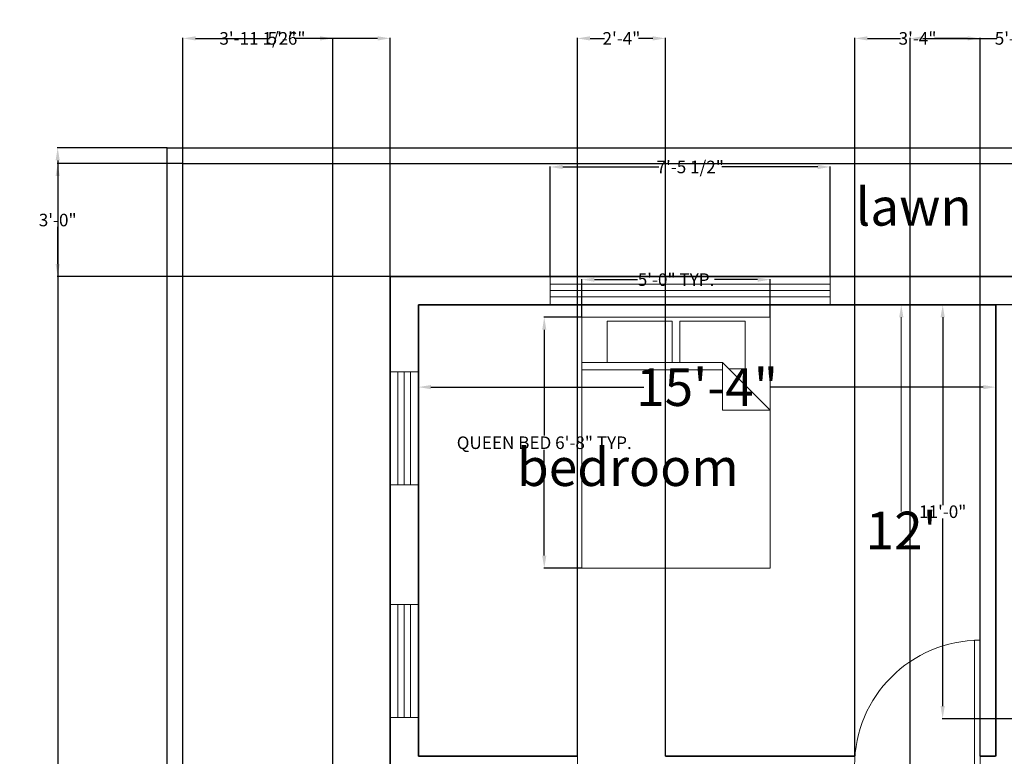
# Model space of a CAD drawing. Units: inches. Extents: x -346 to 220, y 97 to 877.
# Tile 3 of 4: x -346 to -32, y 642 to 877. Entities that reach past the tile are written whole.
import ezdxf

# ---------------------------------------------------------------- set-up
doc = ezdxf.new("R2010")
doc.units = ezdxf.units.IN
doc.header["$MEASUREMENT"] = 0
doc.layers.get('0').update_dxf_attribs({"color": 3})
for name, color, linetype, lineweight in [('A-AREA-IDEN', 130, 'Continuous', 25), ('A-FURN', 8, 'Continuous', 18), ('A-WALL', 7, 'Continuous', 35), ('C-PROP', 94, 'Continuous', 25), ('dim', 170, 'Continuous', 13), ('door', 20, 'Continuous', 18), ('window', 230, 'Continuous', 18)]:
    doc.layers.add(name, color=color, linetype=linetype, lineweight=lineweight)
doc.styles.get("Standard").update_dxf_attribs({"font": 'arial.ttf'})
doc.dimstyles.get("Standard").update_dxf_attribs({"dimtxt": 4, "dimasz": 4, "dimexe": 0.18, "dimexo": 0.0625, "dimgap": 0.09, "dimtad": 0, "dimtih": 1, "dimtoh": 1, "dimdec": 0, "dimzin": 0, "dimdsep": 46, "dimlunit": 3, "dimtxsty": 'Standard', "dimcen": 0.09, "dimadec": 0, "dimazin": 0, "dimtfac": 1, "dimtdec": 0, "dimtofl": 0, "dimtmove": 0, "dimatfit": 3, "dimfxl": 1, "dimtolj": 1, "dimtzin": 0, "dimarcsym": 0})

# ---------------------------------------------------------------- blocks, each defined once
blk = doc.blocks.new('*D1')
at = {"layer": 'Defpoints', "color": 0, "transparency": 16777216}
for p in [(-218.93, 785.75), (-34.93, 785.75), (-34.93, 759.47)]:
    blk.add_point(p, dxfattribs=at)
at = {"layer": 'dim', "color": 0, "lineweight": -2, "transparency": 16777216}
for p, q in [((-218.93, 785.68), (-218.93, 759.29)), ((-34.93, 785.68), (-34.93, 759.29)), ((-214.93, 759.47), (-147.06, 759.47)), ((-38.93, 759.47), (-106.79, 759.47))]:
    blk.add_line(p, q, dxfattribs=at)
at = {"layer": 'dim', "color": 0, "transparency": 16777216}
for points in [[(-214.93, 760.14), (-214.93, 758.8), (-218.93, 759.47)], [(-38.93, 760.14), (-38.93, 758.8), (-34.93, 759.47)]]:
    blk.add_solid(points, dxfattribs=at)
at = {"layer": 'dim', "color": 0, "transparency": 16777216, "insert": (-126.93, 759.47), "char_height": 4, "attachment_point": 5}
blk.add_mtext('\\A1;{\\H3x;15\'-4"}', dxfattribs=at)
blk = doc.blocks.new('*U18')
for p, q in [((0, 0), (0, -6)), ((-40, 0), (-40, -6))]:
    blk.add_line(p, q)
blk.add_lwpolyline([(0, 0), (0, 40), (-1.75, 40), (-1.75, 0)], close=True)
blk.add_arc((0, 0), 40, 90, 180)
blk = doc.blocks.new('Bed - Queen')
for p, q in [((0, -80.00003), (0, 0)), ((0, 0), (59.99999, 0)), ((59.99999, 0), (59.99999, -80.00003)), ((7.99999, -1.2), (28.79998, -1.2)), ((7.99999, -14.4), (7.99999, -1.2)), ((28.79998, -1.2), (28.79998, -14.4)), ((31.19999, -1.2), (51.99999, -1.2)), ((31.19999, -14.4), (31.19999, -1.2)), ((51.99999, -1.2), (51.99999, -16.4)), ((0, -14.4), (44.8, -14.4)), ((59.99999, -29.6), (44.8, -14.4)), ((44.8, -14.4), (44.8, -29.6)), ((44.8, -16.8), (0, -16.8)), ((51.99999, -16.4), (46.79936, -16.4)), ((44.8, -29.6), (59.99999, -29.6)), ((59.99999, -80.00003), (0, -80.00003))]:
    blk.add_line(p, q)
blk = doc.blocks.new('WIN-36x9-PLAN')
for p, q in [((2.5, 36), (2.5, 0)), ((4.5, 36), (4.5, 0)), ((6.5, 36), (6.5, 0))]:
    blk.add_line(p, q)
blk.add_lwpolyline([(0, 36), (9, 36), (9, 0), (0, 0)], close=True)
blk = doc.blocks.new('*D34')
at = {"layer": 'Defpoints', "color": 0, "transparency": 16777216}
for p in [(-178.82, 781.74), (-166.82, 781.74), (-166.82, 701.74)]:
    blk.add_point(p, dxfattribs=at)
at = {"layer": 'dim', "color": 0, "lineweight": -2, "transparency": 16777216}
for p, q in [((-166.88, 781.74), (-179, 781.74)), ((-178.82, 777.74), (-178.82, 744.02)), ((-178.82, 705.74), (-178.82, 739.46)), ((-166.88, 701.74), (-179, 701.74))]:
    blk.add_line(p, q, dxfattribs=at)
at = {"layer": 'dim', "color": 0, "transparency": 16777216}
for points in [[(-179.48, 777.74), (-178.15, 777.74), (-178.82, 781.74)], [(-179.48, 705.74), (-178.15, 705.74), (-178.82, 701.74)]]:
    blk.add_solid(points, dxfattribs=at)
at = {"layer": 'dim', "color": 0, "transparency": 16777216, "insert": (-178.82, 741.74), "char_height": 4, "attachment_point": 5}
blk.add_mtext('\\A1;QUEEN BED 6\'-8" TYP.', dxfattribs=at)
blk = doc.blocks.new('*D35')
at = {"layer": 'Defpoints', "color": 0, "transparency": 16777216}
for p in [(-106.82, 793.74), (-166.82, 781.74), (-106.82, 781.74)]:
    blk.add_point(p, dxfattribs=at)
at = {"layer": 'dim', "color": 0, "lineweight": -2, "transparency": 16777216}
for p, q in [((-166.82, 781.8), (-166.82, 793.92)), ((-106.82, 781.8), (-106.82, 793.92)), ((-162.82, 793.74), (-149.1, 793.74)), ((-110.82, 793.74), (-124.54, 793.74))]:
    blk.add_line(p, q, dxfattribs=at)
at = {"layer": 'dim', "color": 0, "transparency": 16777216}
for points in [[(-162.82, 794.4), (-162.82, 793.07), (-166.82, 793.74)], [(-110.82, 794.4), (-110.82, 793.07), (-106.82, 793.74)]]:
    blk.add_solid(points, dxfattribs=at)
at = {"layer": 'dim', "color": 0, "transparency": 16777216, "insert": (-136.82, 793.74), "char_height": 4, "attachment_point": 5}
blk.add_mtext('\\A1;5\'-0" TYP.', dxfattribs=at)
blk = doc.blocks.new('*D40')
at = {"layer": 'Defpoints', "color": 0, "transparency": 16777216}
for p in [(-93.45, 636.11), (-118, 632.43), (-93.45, 632.43)]:
    blk.add_point(p, dxfattribs=at)
at = {"layer": 'dim', "color": 0, "lineweight": -2, "transparency": 16777216}
for p, q in [((-118, 632.49), (-118, 636.29)), ((-114, 636.11), (-97.45, 636.11)), ((-93.45, 632.49), (-93.45, 636.29)), ((-93.45, 636.11), (-89.45, 636.11))]:
    blk.add_line(p, q, dxfattribs=at)
at = {"layer": 'dim', "color": 0, "transparency": 16777216}
for points in [[(-114, 636.78), (-114, 635.45), (-118, 636.11)], [(-97.45, 636.78), (-97.45, 635.45), (-93.45, 636.11)]]:
    blk.add_solid(points, dxfattribs=at)
at = {"layer": 'dim', "color": 0, "transparency": 16777216, "insert": (-63.43, 636.11), "char_height": 4, "attachment_point": 5}
blk.add_mtext('\\A1;BASIN 2\'-0 1/2" TYP.', dxfattribs=at)
blk = doc.blocks.new('*D49')
at = {"layer": 'Defpoints', "color": 0, "transparency": 16777216}
for p in [(-333.87, 835.75), (-298.95, 835.75), (-298.95, 138.35)]:
    blk.add_point(p, dxfattribs=at)
at = {"layer": 'dim', "color": 0, "lineweight": -2, "transparency": 16777216}
for p, q in [((-299.01, 835.75), (-334.05, 835.75)), ((-333.87, 831.75), (-333.87, 489.21)), ((-333.87, 142.35), (-333.87, 484.89)), ((-299.01, 138.35), (-334.05, 138.35))]:
    blk.add_line(p, q, dxfattribs=at)
at = {"layer": 'dim', "color": 0, "transparency": 16777216}
for points in [[(-334.54, 831.75), (-333.21, 831.75), (-333.87, 835.75)], [(-334.54, 142.35), (-333.21, 142.35), (-333.87, 138.35)]]:
    blk.add_solid(points, dxfattribs=at)
at = {"layer": 'dim', "color": 0, "transparency": 16777216, "insert": (-333.87, 487.05), "char_height": 4, "attachment_point": 5}
blk.add_mtext('\\A1;58\'-1 1/2"', dxfattribs=at)
blk = doc.blocks.new('*D52')
at = {"layer": 'Defpoints', "color": 0, "transparency": 16777216}
for p in [(-246.23, 870.67), (-246.23, 242.75), (-293.95, 143.35)]:
    blk.add_point(p, dxfattribs=at)
at = {"layer": 'dim', "color": 0, "lineweight": -2, "transparency": 16777216}
for p, q in [((-293.95, 143.41), (-293.95, 870.85)), ((-289.95, 870.67), (-281.71, 870.67)), ((-250.23, 870.67), (-258.47, 870.67)), ((-246.23, 242.81), (-246.23, 870.85))]:
    blk.add_line(p, q, dxfattribs=at)
at = {"layer": 'dim', "color": 0, "transparency": 16777216}
for points in [[(-289.95, 871.34), (-289.95, 870), (-293.95, 870.67)], [(-250.23, 871.34), (-250.23, 870), (-246.23, 870.67)]]:
    blk.add_solid(points, dxfattribs=at)
at = {"layer": 'dim', "color": 0, "transparency": 16777216, "insert": (-270.09, 870.67), "char_height": 4, "attachment_point": 5}
blk.add_mtext('\\A1;3\'-11 1/2"', dxfattribs=at)
blk = doc.blocks.new('*D54')
at = {"layer": 'Defpoints', "color": 0, "transparency": 16777216}
for p in [(-293.95, 830.75), (-333.87, 794.75), (-227.93, 794.75)]:
    blk.add_point(p, dxfattribs=at)
at = {"layer": 'dim', "color": 0, "lineweight": -2, "transparency": 16777216}
for p, q in [((-294.01, 830.75), (-334.05, 830.75)), ((-333.87, 826.75), (-333.87, 814.88)), ((-333.87, 798.75), (-333.87, 810.61)), ((-227.99, 794.75), (-334.05, 794.75))]:
    blk.add_line(p, q, dxfattribs=at)
at = {"layer": 'dim', "color": 0, "transparency": 16777216}
for points in [[(-334.54, 826.75), (-333.21, 826.75), (-333.87, 830.75)], [(-334.54, 798.75), (-333.21, 798.75), (-333.87, 794.75)]]:
    blk.add_solid(points, dxfattribs=at)
at = {"layer": 'dim', "color": 0, "transparency": 16777216, "insert": (-333.87, 812.75), "char_height": 4, "attachment_point": 5}
blk.add_mtext('\\A1;3\'-0"', dxfattribs=at)
blk = doc.blocks.new('*D55')
at = {"layer": 'Defpoints', "color": 0, "transparency": 16777216}
for p in [(-227.93, 870.67), (-293.95, 830.75), (-227.93, 794.75)]:
    blk.add_point(p, dxfattribs=at)
at = {"layer": 'dim', "color": 0, "lineweight": -2, "transparency": 16777216}
for p, q in [((-293.95, 830.81), (-293.95, 870.85)), ((-289.95, 870.67), (-266.35, 870.67)), ((-231.93, 870.67), (-255.53, 870.67)), ((-227.93, 794.81), (-227.93, 870.85))]:
    blk.add_line(p, q, dxfattribs=at)
at = {"layer": 'dim', "color": 0, "transparency": 16777216}
for points in [[(-289.95, 871.34), (-289.95, 870), (-293.95, 870.67)], [(-231.93, 871.34), (-231.93, 870), (-227.93, 870.67)]]:
    blk.add_solid(points, dxfattribs=at)
at = {"layer": 'dim', "color": 0, "transparency": 16777216, "insert": (-260.94, 870.67), "char_height": 4, "attachment_point": 5}
blk.add_mtext('\\A1;5\'-6"', dxfattribs=at)
blk = doc.blocks.new('*D56')
at = {"layer": 'Defpoints', "color": 0, "transparency": 16777216}
for p in [(-51.85, 785.75), (-16.93, 785.75), (-16.93, 653.75)]:
    blk.add_point(p, dxfattribs=at)
at = {"layer": 'dim', "color": 0, "lineweight": -2, "transparency": 16777216}
for p, q in [((-16.99, 785.75), (-52.03, 785.75)), ((-51.85, 781.75), (-51.85, 721.88)), ((-51.85, 657.75), (-51.85, 717.61)), ((-16.99, 653.75), (-52.03, 653.75))]:
    blk.add_line(p, q, dxfattribs=at)
at = {"layer": 'dim', "color": 0, "transparency": 16777216}
for points in [[(-52.52, 781.75), (-51.19, 781.75), (-51.85, 785.75)], [(-52.52, 657.75), (-51.19, 657.75), (-51.85, 653.75)]]:
    blk.add_solid(points, dxfattribs=at)
at = {"layer": 'dim', "color": 0, "transparency": 16777216, "insert": (-51.85, 719.75), "char_height": 4, "attachment_point": 5}
blk.add_mtext('\\A1;11\'-0"', dxfattribs=at)
blk = doc.blocks.new('*D58')
at = {"layer": 'Defpoints', "color": 0, "transparency": 16777216}
for p in [(3.77, 870.67), (3.77, 341.75), (-62.23, 331.75)]:
    blk.add_point(p, dxfattribs=at)
at = {"layer": 'dim', "color": 0, "lineweight": -2, "transparency": 16777216}
for p, q in [((-62.23, 331.81), (-62.23, 870.85)), ((-58.23, 870.67), (-34.63, 870.67)), ((-0.23, 870.67), (-23.82, 870.67)), ((3.77, 341.81), (3.77, 870.85))]:
    blk.add_line(p, q, dxfattribs=at)
at = {"layer": 'dim', "color": 0, "transparency": 16777216}
for points in [[(-58.23, 871.34), (-58.23, 870), (-62.23, 870.67)], [(-0.23, 871.34), (-0.23, 870), (3.77, 870.67)]]:
    blk.add_solid(points, dxfattribs=at)
at = {"layer": 'dim', "color": 0, "transparency": 16777216, "insert": (-29.23, 870.67), "char_height": 4, "attachment_point": 5}
blk.add_mtext('\\A1;5\'-6"', dxfattribs=at)
blk = doc.blocks.new('*D62')
at = {"layer": 'Defpoints', "color": 0, "transparency": 16777216}
for p in [(-140.23, 870.67), (-168.23, 641.75), (-140.23, 641.75)]:
    blk.add_point(p, dxfattribs=at)
at = {"layer": 'dim', "color": 0, "lineweight": -2, "transparency": 16777216}
for p, q in [((-168.23, 641.81), (-168.23, 870.85)), ((-164.23, 870.67), (-159.67, 870.67)), ((-144.23, 870.67), (-148.79, 870.67)), ((-140.23, 641.81), (-140.23, 870.85))]:
    blk.add_line(p, q, dxfattribs=at)
at = {"layer": 'dim', "color": 0, "transparency": 16777216}
for points in [[(-164.23, 871.34), (-164.23, 870), (-168.23, 870.67)], [(-144.23, 871.34), (-144.23, 870), (-140.23, 870.67)]]:
    blk.add_solid(points, dxfattribs=at)
at = {"layer": 'dim', "color": 0, "transparency": 16777216, "insert": (-154.23, 870.67), "char_height": 4, "attachment_point": 5}
blk.add_mtext('\\A1;2\'-4"', dxfattribs=at)
blk = doc.blocks.new('*D64')
at = {"layer": 'Defpoints', "color": 0, "transparency": 16777216}
for p in [(-39.93, 870.67), (-79.82, 641.75), (-39.93, 641.75)]:
    blk.add_point(p, dxfattribs=at)
at = {"layer": 'dim', "color": 0, "lineweight": -2, "transparency": 16777216}
for p, q in [((-79.82, 641.81), (-79.82, 870.85)), ((-75.82, 870.67), (-65.28, 870.67)), ((-43.93, 870.67), (-54.47, 870.67)), ((-39.93, 641.81), (-39.93, 870.85))]:
    blk.add_line(p, q, dxfattribs=at)
at = {"layer": 'dim', "color": 0, "transparency": 16777216}
for points in [[(-75.82, 871.34), (-75.82, 870), (-79.82, 870.67)], [(-43.93, 871.34), (-43.93, 870), (-39.93, 870.67)]]:
    blk.add_solid(points, dxfattribs=at)
at = {"layer": 'dim', "color": 0, "transparency": 16777216, "insert": (-59.87, 870.67), "char_height": 4, "attachment_point": 5}
blk.add_mtext('\\A1;3\'-4"', dxfattribs=at)
blk = doc.blocks.new('*D69')
at = {"layer": 'Defpoints', "color": 0, "transparency": 16777216}
for p in [(-87.66, 829.67), (-176.95, 794.75), (-87.66, 794.75)]:
    blk.add_point(p, dxfattribs=at)
at = {"layer": 'dim', "color": 0, "lineweight": -2, "transparency": 16777216}
for p, q in [((-176.95, 794.81), (-176.95, 829.85)), ((-172.95, 829.67), (-142.35, 829.67)), ((-91.66, 829.67), (-122.25, 829.67)), ((-87.66, 794.81), (-87.66, 829.85))]:
    blk.add_line(p, q, dxfattribs=at)
at = {"layer": 'dim', "color": 0, "transparency": 16777216}
for points in [[(-172.95, 830.34), (-172.95, 829), (-176.95, 829.67)], [(-91.66, 830.34), (-91.66, 829), (-87.66, 829.67)]]:
    blk.add_solid(points, dxfattribs=at)
at = {"layer": 'dim', "color": 0, "transparency": 16777216, "insert": (-132.3, 829.67), "char_height": 4, "attachment_point": 5}
blk.add_mtext('\\A1;7\'-5 1/2"', dxfattribs=at)

msp = doc.modelspace()

# ---------------------------------------------------------------- linework, layer by layer
at = {"layer": 'A-WALL'}
for p, q in [((-227.93, 632.75), (-227.93, 794.75)), ((-227.93, 794.75), (93.07, 794.75)), ((-218.93, 785.75), (-34.93, 785.75)), ((-218.93, 641.75), (-218.93, 785.75)), ((-34.93, 785.75), (-34.93, 641.75)), ((-168.23, 641.75), (-218.93, 641.75)), ((-79.82, 641.75), (-140.23, 641.75)), ((-34.99, 641.75), (-39.93, 641.75))]:
    msp.add_line(p, q, dxfattribs=at)
at = {"layer": 'C-PROP'}
for p, q in [((-298.95, 835.75), (177.07, 835.75)), ((-298.95, 138.35), (-298.95, 835.75)), ((-293.95, 830.75), (84.07, 830.75)), ((-293.95, 143.35), (-293.95, 830.75))]:
    msp.add_line(p, q, dxfattribs=at)
at = {"layer": 'dim'}
for p, q in [((-34.99, 785.75), (-65.23, 785.75)), ((-65.05, 781.75), (-65.05, 719.86))]:
    msp.add_line(p, q, dxfattribs=at)
msp.add_solid([(-65.71, 781.75), (-64.38, 781.75), (-65.05, 785.75)], dxfattribs=at)
at = {"layer": 'door'}
for p, q in [((-168.23, 632.68), (-168.23, 641.75)), ((-39.93, 641.75), (-39.93, 632.75))]:
    msp.add_line(p, q, dxfattribs=at)
at = {"layer": 'window'}
for p, q in [((-176.95, 794.75), (-176.95, 785.75)), ((-87.66, 794.75), (-87.66, 785.75)), ((-87.66, 792.25), (-176.93, 792.25)), ((-87.66, 790.25), (-176.93, 790.25)), ((-87.66, 788.25), (-176.93, 788.25))]:
    msp.add_line(p, q, dxfattribs=at)

# ---------------------------------------------------------------- block references
at = {"layer": 'A-FURN'}
msp.add_blockref('Bed - Queen', (-166.82, 781.74), dxfattribs=at)
at = {"layer": 'door'}
msp.add_blockref('*U18', (-39.93, 638.75), dxfattribs=at)
at = {"layer": 'window'}
for p in [(-227.95, 728.31), (-227.95, 654.11)]:
    msp.add_blockref('WIN-36x9-PLAN', p, dxfattribs=at)

# ---------------------------------------------------------------- texts
at = {"layer": 'A-AREA-IDEN', "char_height": 12, "attachment_point": 1}
for s, width, insert in [(' lawn', 179.6897, (-83.24, 822.96)), ('bedroom', 62.6765, (-187.5, 739.94))]:
    msp.add_mtext_dynamic_manual_height_columns(s, width=width, gutter_width=1, heights=[0], dxfattribs=dict(at, insert=insert))
at = {"layer": 'dim', "insert": (-65.05, 713.75), "char_height": 4, "attachment_point": 5}
msp.add_mtext("\\A1;{\\H3x;12'}", dxfattribs=at)

# ---------------------------------------------------------------- dimensions: what is measured, and where the dimension line sits
at = {"layer": 'dim'}
for base, p1, p2, picture, middle in [((-246.23, 870.67), (-293.95, 143.35), (-246.23, 242.75), '*D52', (-270.09, 870.67)), ((-227.93, 870.67), (-293.95, 830.75), (-227.93, 794.75), '*D55', (-260.94, 870.67)), ((-140.23, 870.67), (-168.23, 641.75), (-140.23, 641.75), '*D62', (-154.23, 870.67)), ((-39.93, 870.67), (-79.82, 641.75), (-39.93, 641.75), '*D64', (-59.87, 870.67)), ((3.77, 870.67), (-62.23, 331.75), (3.77, 341.75), '*D58', (-29.23, 870.67)), ((-87.66, 829.67), (-176.95, 794.75), (-87.66, 794.75), '*D69', (-132.3, 829.67))]:
    dim = msp.add_linear_dim(base=base, p1=p1, p2=p2, dimstyle='Standard', override={"dimdec": 1, "dimlfac": 1, "dimrnd": 0, "dimzin": 1, "dimdsep": 46, "dimlunit": 4, "dimfrac": 2}, dxfattribs=at)
    dim.commit()
    dim.dimension.update_dxf_attribs({"geometry": picture, "text_midpoint": middle})
for base, p1, p2, picture, middle in [((-333.87, 835.75), (-298.95, 138.35), (-298.95, 835.75), '*D49', (-333.87, 487.05)), ((-333.87, 794.75), (-293.95, 830.75), (-227.93, 794.75), '*D54', (-333.87, 812.75)), ((-51.85, 785.75), (-16.93, 653.75), (-16.93, 785.75), '*D56', (-51.85, 719.75))]:
    dim = msp.add_linear_dim(base=base, p1=p1, p2=p2, angle=90, dimstyle='Standard', override={"dimdec": 1, "dimlfac": 1, "dimrnd": 0, "dimzin": 1, "dimdsep": 46, "dimlunit": 4, "dimfrac": 2}, dxfattribs=at)
    dim.commit()
    dim.dimension.update_dxf_attribs({"geometry": picture, "text_midpoint": middle})
for base, p1, p2, text, override, picture, middle in [((-106.82, 793.74), (-166.82, 781.74), (-106.82, 781.74), '<> TYP.', {"dimdec": 1, "dimlfac": 1, "dimrnd": 0, "dimzin": 1, "dimdsep": 46, "dimlunit": 4, "dimfrac": 2}, '*D35', (-136.82, 793.74)), ((-34.93, 759.47), (-218.93, 785.75), (-34.93, 785.75), '{\\H3x;<>}', {"dimclrd": 0, "dimclre": 0, "dimclrt": 0}, '*D1', (-126.93, 759.47)), ((-93.4485, 636.1143), (-117.9994, 632.4317), (-93.4485, 632.4317), 'BASIN <> TYP.', {"dimdec": 1, "dimlfac": 1, "dimrnd": 0, "dimzin": 1, "dimdsep": 46, "dimlunit": 4, "dimfrac": 2}, '*D40', (-63.4349, 636.1143))]:
    dim = msp.add_linear_dim(base=base, p1=p1, p2=p2, text=text, dimstyle='Standard', override=override, dxfattribs=at)
    dim.commit()
    dim.dimension.update_dxf_attribs({"geometry": picture, "text_midpoint": middle})
dim = msp.add_linear_dim(base=(-178.82, 781.74), p1=(-166.82, 701.74), p2=(-166.82, 781.74), angle=90, text='QUEEN BED <> TYP.', dimstyle='Standard', override={"dimdec": 1, "dimlfac": 1, "dimrnd": 0, "dimzin": 1, "dimdsep": 46, "dimlunit": 4, "dimfrac": 2}, dxfattribs=at)
dim.commit()
dim.dimension.update_dxf_attribs({"geometry": '*D34', "text_midpoint": (-178.82, 741.74)})

doc.saveas('drawing.dxf')
